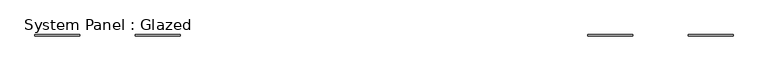
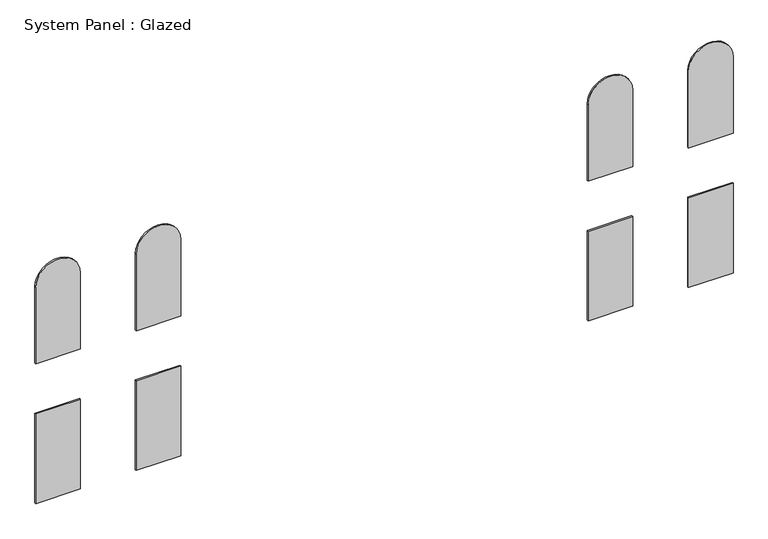
"""IFC4 building model written with IfcOpenShell, lengths in millimetres: plate geometry, System Panel : Glazed."""

from ifc_helpers import new_model, si_unit, point, frame, frame_2d, origin, origin_with_axes, place, context, project, spatial, polyline, circle_curve, trimmed, segment, composite_curve, outline, extrude, source, transform, mapped, element, save


def system_panel_glazed_d30904ce(model_context):
    return source(origin(), model_context, "Body", "SweptSolid", [
        extrude(outline(composite_curve([segment(polyline([(2692.4, 5537.2), (2692.4, 6350.0), (4165.6, 6350.0)]), True, "CONTINUOUS"), segment(trimmed(circle_curve(frame_2d((4165.6, 5943.6)), 406.4), [point((4165.6, 6350.0))], [point((4165.6, 5537.2))], False, "CARTESIAN"), True, "CONTINUOUS"), segment(polyline([(4165.6, 5537.2), (2692.4, 5537.2)]), True, "CONTINUOUS")], self_intersect=False)), frame((0.0, 19.05, 0.0), z_axis=(0.0, 1.0, 0.0), x_axis=(0.0, 0.0, 1.0)), (0.0, 0.0, 1.0), 25.4),
        extrude(outline(polyline([(6350.0, 19.05), (5537.2, 19.05), (5537.2, 44.45), (6350.0, 44.45), (6350.0, 19.05)])), origin_with_axes(), (0.0, 0.0, 1.0), 1727.2),
        extrude(outline(composite_curve([segment(polyline([(2692.4, 3708.4), (2692.4, 4521.2), (4165.6, 4521.2)]), True, "CONTINUOUS"), segment(trimmed(circle_curve(frame_2d((4165.6, 4114.8)), 406.4), [point((4165.6, 4521.2))], [point((4165.6, 3708.4))], False, "CARTESIAN"), True, "CONTINUOUS"), segment(polyline([(4165.6, 3708.4), (2692.4, 3708.4)]), True, "CONTINUOUS")], self_intersect=False)), frame((0.0, 19.05, 0.0), z_axis=(0.0, 1.0, 0.0), x_axis=(0.0, 0.0, 1.0)), (0.0, 0.0, 1.0), 25.4),
        extrude(outline(polyline([(4521.2, 19.05), (3708.4, 19.05), (3708.4, 44.45), (4521.2, 44.45), (4521.2, 19.05)])), origin_with_axes(), (0.0, 0.0, 1.0), 1727.2),
        extrude(outline(composite_curve([segment(polyline([(2692.4, -4521.2), (2692.4, -3708.4), (4165.6, -3708.4)]), True, "CONTINUOUS"), segment(trimmed(circle_curve(frame_2d((4165.6, -4114.8)), 406.4), [point((4165.6, -3708.4))], [point((4165.6, -4521.2))], False, "CARTESIAN"), True, "CONTINUOUS"), segment(polyline([(4165.6, -4521.2), (2692.4, -4521.2)]), True, "CONTINUOUS")], self_intersect=False)), frame((0.0, 19.05, 0.0), z_axis=(0.0, 1.0, 0.0), x_axis=(0.0, 0.0, 1.0)), (0.0, 0.0, 1.0), 25.4),
        extrude(outline(polyline([(-3708.4, 19.05), (-4521.2, 19.05), (-4521.2, 44.45), (-3708.4, 44.45), (-3708.4, 19.05)])), origin_with_axes(), (0.0, 0.0, 1.0), 1727.2),
        extrude(outline(composite_curve([segment(polyline([(2692.4, -6350.0), (2692.4, -5537.2), (4165.6, -5537.2)]), True, "CONTINUOUS"), segment(trimmed(circle_curve(frame_2d((4165.6, -5943.6)), 406.4), [point((4165.6, -5537.2))], [point((4165.6, -6350.0))], False, "CARTESIAN"), True, "CONTINUOUS"), segment(polyline([(4165.6, -6350.0), (2692.4, -6350.0)]), True, "CONTINUOUS")], self_intersect=False)), frame((0.0, 19.05, 0.0), z_axis=(0.0, 1.0, 0.0), x_axis=(0.0, 0.0, 1.0)), (0.0, 0.0, 1.0), 25.4),
        extrude(outline(polyline([(-5537.2, 19.05), (-6350.0, 19.05), (-6350.0, 44.45), (-5537.2, 44.45), (-5537.2, 19.05)])), origin_with_axes(), (0.0, 0.0, 1.0), 1727.2),
    ])


if __name__ == "__main__":
    model = new_model("IFC4")
    model_context = context("Model", 3, world=origin())
    ifc_project = project(units=[si_unit("LENGTHUNIT", "METRE", prefix="MILLI")], contexts=[model_context])
    site = spatial("IfcSite", under=ifc_project)
    building = spatial("IfcBuilding", under=site)
    placement = place(None, origin())
    system_panel_glazed_shape = system_panel_glazed_d30904ce(model_context)
    element("IfcPlate", 1, ObjectType="System Panel : Glazed", at=placement, inside=building, context=model_context, shape_type="MappedRepresentation", body=[
        mapped(system_panel_glazed_shape, transform((0.0, 0.0, 0.0), x_axis=(1.0, 0.0, 0.0), y_axis=(0.0, 1.0, 0.0), z_axis=(0.0, 0.0, 1.0))),
    ])
    save(model, "model.ifc")

# Revit data of these elements
# Type "System Panel : Glazed"
#   Construction Type Id = "GSP4R"
#   Analytic Construction = "1/8 in Pilkington single glazing"
#   Visual Light Transmittance = 0.9
#   Solar Heat Gain Coefficient = 0.86
#   Heat Transfer Coefficient (U) = 1.18115 BTU/(h·ft²·°F)
#   Define Thermal Properties by = 1
# Element 1 (IfcPlate, "System Panel : Glazed")
#   Materials on its faces: "Glass"
# Materials
#   "Glass": class "Glass", colour RGB 245 245 243, transparency 1, Description = "Soda Lime Glass", Cost = 0
